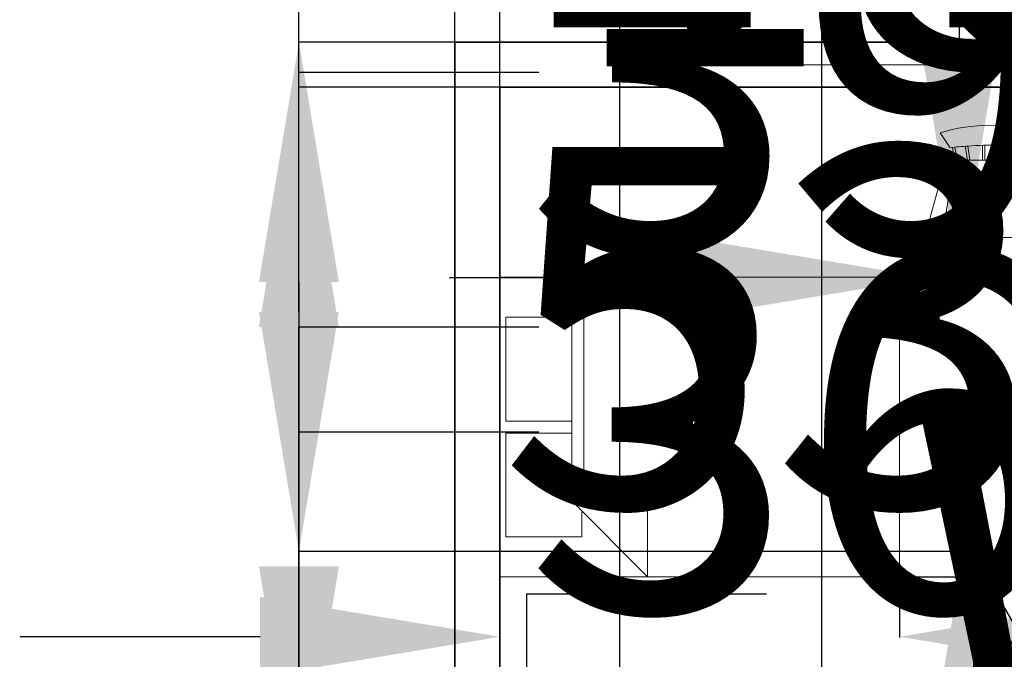
# Model space of a CAD drawing. Units: inches. Extents: x -307 to 2141, y -58 to 895.
# Tile 11 of 28: x 469 to 666, y 568 to 696. Entities that reach past the tile are written whole.
import ezdxf

# ---------------------------------------------------------------- set-up
doc = ezdxf.new("R2010")
doc.units = ezdxf.units.IN
doc.header["$MEASUREMENT"] = 0
for name, color, linetype, lineweight in [('A-ANNO-DIMS', 2, 'Continuous', 18), ('A-DOOR', 3, 'Continuous', 25), ('A-FURN', 8, 'Continuous', 18), ('A-GLAZ', 4, 'Continuous', 18), ('A-WALL', 7, 'Continuous', 35)]:
    doc.layers.add(name, color=color, linetype=linetype, lineweight=lineweight)
doc.styles.get("Standard").update_dxf_attribs({"font": 'arial.ttf'})
doc.dimstyles.get("Standard").update_dxf_attribs({"dimtxt": 72, "dimasz": 48, "dimexe": 0.18, "dimexo": 0.0625, "dimgap": 0.09, "dimtad": 0, "dimtih": 1, "dimtoh": 1, "dimdec": 0, "dimrnd": 48, "dimzin": 0, "dimdsep": 46, "dimlunit": 3, "dimtxsty": 'Standard', "dimcen": 0.09, "dimadec": 0, "dimazin": 0, "dimtfac": 1, "dimtdec": 0, "dimtofl": 0, "dimtmove": 0, "dimatfit": 3, "dimfxl": 1, "dimtolj": 1, "dimtzin": 0, "dimarcsym": 0})

# ---------------------------------------------------------------- blocks, each defined once
blk = doc.blocks.new('*U3')
for p, q in [((-40, 0), (-40, 6)), ((0, 0), (0, 6))]:
    blk.add_line(p, q)
blk.add_lwpolyline([(0, 0), (-34.64, -20), (-35.52, -18.48), (-0.88, 1.52)], close=True)
blk.add_arc((0, 0), 40, 180, 210)
blk = doc.blocks.new('Chair - Rocking')
for p, q in [((-8, -4.5), (-10, -1.5)), ((8, -4.5), (10, -1.5)), ((-7.5, -4.5), (-7, -7)), ((-6.5, -7), (-7.02225, -4.43)), ((-4.5, -7), (-4.96674, -4.19951)), ((-4, -7), (-4.40532, -4.16272)), ((-1.5, -4.05012), (-1.5, -7)), ((-1, -7), (-1, -4.05012)), ((1, -7), (1, -4.04655)), ((1.5, -4.05012), (1.5, -7)), ((4, -7), (4.40187, -4.18694)), ((4.5, -7), (4.96761, -4.19437)), ((6.5, -7), (7, -4.4057)), ((7.5, -4.5), (7, -7)), ((-9, -7.5), (-12, -18.49999)), ((-7, -7.5), (-9, -7.5)), ((-9, -18.49999), (-7, -7.5)), ((-8.23428, -6.99939), (-8.3093, -7.47958)), ((-8.23041, -7), (8.23915, -7)), ((7, -7.5), (9, -7.5)), ((9, -18.49999), (7, -7.5)), ((8.31071, -7.48854), (8.23449, -7.00073)), ((9, -7.5), (12, -18.49999)), ((-10.36644, -20.64523), (-10.5, -21.49999)), ((10.5, -21.49999), (10.3575, -20.58798)), ((-9, -22.49999), (-9.5, -26.49999)), ((0, -22.49999), (-9.5, -22.49999)), ((-8, -26.49999), (-7.5, -22.49999)), ((0, -22.49999), (9.5, -22.49999)), ((8, -26.49999), (7.5, -22.49999)), ((9, -22.49999), (9.5, -26.49999)), ((-9.5, -26.49999), (-8, -26.49999)), ((9.5, -26.49999), (8, -26.49999))]:
    blk.add_line(p, q)
for centre, radius, start, end in [((0, -34.08333), 34.08333, 72.93847, 107.0615), ((0, -68.25004), 64.25, 93.92211, 97.15267), ((0, -68.25004), 64.25, 82.84733, 93.92211), ((-10.5, -18.99999), 1.58114, 161.5651, 18.43495), ((10.5, -18.99999), 1.58114, 161.5651, 18.43495), ((-9.5, -21.49999), 1, 180, 270), ((9.5, -21.49999), 1, 270, 0)]:
    blk.add_arc(centre, radius, start, end)
blk = doc.blocks.new('Bed - Queen')
for p, q in [((0, -80.00003), (0, 0)), ((0, 0), (59.99999, 0)), ((59.99999, 0), (59.99999, -80.00003)), ((7.99999, -1.2), (28.79998, -1.2)), ((7.99999, -14.4), (7.99999, -1.2)), ((28.79998, -1.2), (28.79998, -14.4)), ((31.19999, -1.2), (51.99999, -1.2)), ((31.19999, -14.4), (31.19999, -1.2)), ((51.99999, -1.2), (51.99999, -16.4)), ((0, -14.4), (44.8, -14.4)), ((59.99999, -29.6), (44.8, -14.4)), ((44.8, -14.4), (44.8, -29.6)), ((44.8, -16.8), (0, -16.8)), ((51.99999, -16.4), (46.79936, -16.4)), ((44.8, -29.6), (59.99999, -29.6)), ((59.99999, -80.00003), (0, -80.00003))]:
    blk.add_line(p, q)
blk = doc.blocks.new('WIN-72IN')
blk.add_line((72, 4.5), (0, 4.5))
blk.add_lwpolyline([(72, 0), (0, 0), (0, 9), (72, 9)], close=True)
blk = doc.blocks.new('*D26')
at = {"layer": 'A-ANNO-DIMS', "color": 0, "lineweight": -2, "transparency": 16777216}
for p, q in [((565.34, 584.2), (565.34, 572.08)), ((645.34, 584.2), (645.34, 572.08)), ((517.34, 572.26), (469.34, 572.26)), ((693.34, 572.26), (741.34, 572.26))]:
    blk.add_line(p, q, dxfattribs=at)
at = {"layer": 'A-ANNO-DIMS', "color": 0, "transparency": 16777216}
for points in [[(517.34, 580.26), (517.34, 564.26), (565.34, 572.26)], [(693.34, 580.26), (693.34, 564.26), (645.34, 572.26)]]:
    blk.add_solid(points, dxfattribs=at)
at = {"layer": 'Defpoints', "color": 0, "transparency": 16777216}
for p in [(565.34, 584.26), (645.34, 584.26), (565.34, 572.26)]:
    blk.add_point(p, dxfattribs=at)
at = {"layer": 'A-ANNO-DIMS', "color": 0, "transparency": 16777216, "insert": (178.23, 572.26), "char_height": 72, "attachment_point": 5}
blk.add_mtext('\\A1;BED 80 TYP.', dxfattribs=at)
blk = doc.blocks.new('*D27')
at = {"layer": 'A-ANNO-DIMS', "color": 0, "lineweight": -2, "transparency": 16777216}
for p, q in [((657.34, 692.26), (657.34, 740.26)), ((645.4, 644.26), (657.52, 644.26)), ((645.4, 584.26), (657.52, 584.26)), ((657.34, 536.26), (657.34, 488.26)), ((657.34, 488.26), (609.34, 488.26))]:
    blk.add_line(p, q, dxfattribs=at)
at = {"layer": 'A-ANNO-DIMS', "color": 0, "transparency": 16777216}
for points in [[(649.34, 692.26), (665.34, 692.26), (657.34, 644.26)], [(649.34, 536.26), (665.34, 536.26), (657.34, 584.26)]]:
    blk.add_solid(points, dxfattribs=at)
at = {"layer": 'Defpoints', "color": 0, "transparency": 16777216}
for p in [(645.34, 644.26), (645.34, 584.26), (657.34, 584.26)]:
    blk.add_point(p, dxfattribs=at)
at = {"layer": 'A-ANNO-DIMS', "color": 0, "transparency": 16777216, "insert": (433.81, 488.26), "char_height": 72, "attachment_point": 5}
blk.add_mtext('\\A1;60 TYP.', dxfattribs=at)
blk = doc.blocks.new('*D30')
at = {"layer": 'A-ANNO-DIMS', "color": 0, "lineweight": -2, "transparency": 16777216}
for p, q in [((570.74, 532.83), (570.74, 580.83)), ((570.74, 580.83), (618.74, 580.83)), ((565.4, 484.83), (570.92, 484.83)), ((565.4, 448.83), (570.92, 448.83)), ((570.74, 400.83), (570.74, 352.83))]:
    blk.add_line(p, q, dxfattribs=at)
at = {"layer": 'A-ANNO-DIMS', "color": 0, "transparency": 16777216}
for points in [[(562.74, 532.83), (578.74, 532.83), (570.74, 484.83)], [(562.74, 400.83), (578.74, 400.83), (570.74, 448.83)]]:
    blk.add_solid(points, dxfattribs=at)
at = {"layer": 'Defpoints', "color": 0, "transparency": 16777216}
for p in [(565.34, 484.83), (570.74, 484.83), (565.34, 448.83)]:
    blk.add_point(p, dxfattribs=at)
at = {"layer": 'A-ANNO-DIMS', "color": 0, "transparency": 16777216, "insert": (1030.17, 580.83), "char_height": 72, "attachment_point": 5}
blk.add_mtext('\\A1;WINDOW 36 TYP.', dxfattribs=at)
blk = doc.blocks.new('*D36')
at = {"layer": 'A-ANNO-DIMS', "color": 0, "lineweight": -2, "transparency": 16777216}
for p, q in [((871.71, 562.4), (871.76, 610.4)), ((876.55, 514.4), (871.47, 514.4)), ((876.51, 481.35), (871.44, 481.36)), ((871.56, 433.36), (871.51, 385.36)), ((871.51, 385.36), (823.51, 385.36))]:
    blk.add_line(p, q, dxfattribs=at)
at = {"layer": 'A-ANNO-DIMS', "color": 0, "transparency": 16777216}
for points in [[(863.71, 562.41), (879.71, 562.4), (871.65, 514.4)], [(863.56, 433.37), (879.56, 433.35), (871.62, 481.36)]]:
    blk.add_solid(points, dxfattribs=at)
at = {"layer": 'Defpoints', "color": 0, "transparency": 16777216}
for p in [(876.61, 514.4), (871.62, 481.36), (876.57, 481.35)]:
    blk.add_point(p, dxfattribs=at)
at = {"layer": 'A-ANNO-DIMS', "color": 0, "transparency": 16777216, "insert": (548.95, 385.36), "char_height": 72, "attachment_point": 5}
blk.add_mtext('\\A1;WC 33 TYP.', dxfattribs=at)
blk = doc.blocks.new('*D37')
at = {"layer": 'A-ANNO-DIMS', "color": 0, "lineweight": -2, "transparency": 16777216}
for p, q in [((828.62, 519.41), (780.62, 519.46)), ((876.61, 514.46), (876.62, 519.54)), ((897.61, 514.44), (897.62, 519.51)), ((945.62, 519.28), (993.62, 519.22))]:
    blk.add_line(p, q, dxfattribs=at)
at = {"layer": 'A-ANNO-DIMS', "color": 0, "transparency": 16777216}
for points in [[(828.63, 527.41), (828.61, 511.41), (876.62, 519.36)], [(945.63, 527.28), (945.61, 511.28), (897.62, 519.33)]]:
    blk.add_solid(points, dxfattribs=at)
at = {"layer": 'Defpoints', "color": 0, "transparency": 16777216}
for p in [(876.62, 519.36), (876.61, 514.4), (897.61, 514.38)]:
    blk.add_point(p, dxfattribs=at)
at = {"layer": 'A-ANNO-DIMS', "color": 0, "transparency": 16777216, "insert": (604.68, 519.46), "char_height": 72, "attachment_point": 5}
blk.add_mtext('\\A1;21 TYP.', dxfattribs=at)
blk = doc.blocks.new('*D52')
at = {"layer": 'A-ANNO-DIMS', "color": 0, "lineweight": -2, "transparency": 16777216}
for p, q in [((660.21, 554.25), (660.21, 602.25)), ((673.8, 506.25), (660.03, 506.25)), ((673.8, 415.25), (660.03, 415.25)), ((660.21, 367.25), (660.21, 319.25))]:
    blk.add_line(p, q, dxfattribs=at)
at = {"layer": 'A-ANNO-DIMS', "color": 0, "transparency": 16777216}
for points in [[(652.21, 554.25), (668.21, 554.25), (660.21, 506.25)], [(652.21, 367.25), (668.21, 367.25), (660.21, 415.25)]]:
    blk.add_solid(points, dxfattribs=at)
at = {"layer": 'Defpoints', "color": 0, "transparency": 16777216}
for p in [(673.86, 506.25), (660.21, 415.25), (673.86, 415.25)]:
    blk.add_point(p, dxfattribs=at)
at = {"layer": 'A-ANNO-DIMS', "color": 0, "transparency": 16777216, "insert": (660.21, 460.75), "char_height": 72, "attachment_point": 5}
blk.add_mtext('\\A1;DINING SET 91', dxfattribs=at)
blk = doc.blocks.new('*D57')
at = {"layer": 'A-ANNO-DIMS', "color": 0, "lineweight": -2, "transparency": 16777216}
for p, q in [((651.25, 648.15), (651.25, 643.98)), ((675.68, 648.15), (675.68, 643.98)), ((603.25, 644.16), (555.25, 644.16)), ((723.68, 644.16), (771.68, 644.16))]:
    blk.add_line(p, q, dxfattribs=at)
at = {"layer": 'A-ANNO-DIMS', "color": 0, "transparency": 16777216}
for points in [[(603.25, 652.16), (603.25, 636.16), (651.25, 644.16)], [(723.68, 652.16), (723.68, 636.16), (675.68, 644.16)]]:
    blk.add_solid(points, dxfattribs=at)
at = {"layer": 'Defpoints', "color": 0, "transparency": 16777216}
for p in [(651.25, 648.21), (675.68, 648.21), (675.68, 644.16)]:
    blk.add_point(p, dxfattribs=at)
at = {"layer": 'A-ANNO-DIMS', "color": 0, "transparency": 16777216, "insert": (823.81, 644.16), "char_height": 72, "attachment_point": 5}
blk.add_mtext('\\A1;24', dxfattribs=at)
blk = doc.blocks.new('*D62')
at = {"layer": 'A-ANNO-DIMS', "color": 0, "lineweight": -2, "transparency": 16777216}
for p, q in [((556.34, 691.4), (556.34, 722.72)), ((604.34, 722.54), (656.85, 722.54)), ((868.34, 722.54), (815.82, 722.54)), ((916.34, 490.97), (916.34, 722.72))]:
    blk.add_line(p, q, dxfattribs=at)
at = {"layer": 'A-ANNO-DIMS', "color": 0, "transparency": 16777216}
for points in [[(604.34, 730.54), (604.34, 714.54), (556.34, 722.54)], [(868.34, 730.54), (868.34, 714.54), (916.34, 722.54)]]:
    blk.add_solid(points, dxfattribs=at)
at = {"layer": 'Defpoints', "color": 0, "transparency": 16777216}
for p in [(916.34, 722.54), (556.34, 691.34), (916.34, 490.9)]:
    blk.add_point(p, dxfattribs=at)
at = {"layer": 'A-ANNO-DIMS', "color": 0, "transparency": 16777216, "insert": (736.34, 722.54), "char_height": 72, "attachment_point": 5}
blk.add_mtext('\\A1;360', dxfattribs=at)
blk = doc.blocks.new('*D64')
at = {"layer": 'A-ANNO-DIMS', "color": 0, "lineweight": -2, "transparency": 16777216}
for p, q in [((556.27, 691.34), (524.95, 691.34)), ((525.13, 643.34), (525.13, 465.69)), ((525.13, 214.34), (525.13, 391.99)), ((556.27, 166.34), (524.95, 166.34))]:
    blk.add_line(p, q, dxfattribs=at)
at = {"layer": 'A-ANNO-DIMS', "color": 0, "transparency": 16777216}
for points in [[(517.13, 643.34), (533.13, 643.34), (525.13, 691.34)], [(517.13, 214.34), (533.13, 214.34), (525.13, 166.34)]]:
    blk.add_solid(points, dxfattribs=at)
at = {"layer": 'Defpoints', "color": 0, "transparency": 16777216}
for p in [(525.13, 691.34), (556.34, 691.34), (556.34, 166.34)]:
    blk.add_point(p, dxfattribs=at)
at = {"layer": 'A-ANNO-DIMS', "color": 0, "transparency": 16777216, "insert": (525.13, 428.84), "char_height": 72, "attachment_point": 5}
blk.add_mtext('\\A1;525', dxfattribs=at)
blk = doc.blocks.new('*D68')
at = {"layer": 'A-ANNO-DIMS', "color": 0, "lineweight": -2, "transparency": 16777216}
for p, q in [((525.13, 586.34), (525.13, 634.34)), ((525.13, 634.34), (573.13, 634.34)), ((565.27, 538.34), (524.95, 538.34)), ((556.27, 484.83), (524.95, 484.83)), ((525.13, 436.83), (525.13, 388.83))]:
    blk.add_line(p, q, dxfattribs=at)
at = {"layer": 'A-ANNO-DIMS', "color": 0, "transparency": 16777216}
for points in [[(517.13, 586.34), (533.13, 586.34), (525.13, 538.34)], [(517.13, 436.83), (533.13, 436.83), (525.13, 484.83)]]:
    blk.add_solid(points, dxfattribs=at)
at = {"layer": 'Defpoints', "color": 0, "transparency": 16777216}
for p in [(525.13, 538.34), (565.34, 538.34), (556.34, 484.83)]:
    blk.add_point(p, dxfattribs=at)
at = {"layer": 'A-ANNO-DIMS', "color": 0, "transparency": 16777216, "insert": (687.75, 634.34), "char_height": 72, "attachment_point": 5}
blk.add_mtext('\\A1;53.51', dxfattribs=at)
blk = doc.blocks.new('*D69')
at = {"layer": 'A-ANNO-DIMS', "color": 0, "lineweight": -2, "transparency": 16777216}
for p, q in [((525.13, 682.34), (525.13, 730.34)), ((525.13, 730.34), (573.13, 730.34)), ((565.27, 682.34), (524.95, 682.34)), ((525.13, 586.34), (525.13, 634.34)), ((565.27, 538.34), (524.95, 538.34))]:
    blk.add_line(p, q, dxfattribs=at)
at = {"layer": 'A-ANNO-DIMS', "color": 0, "transparency": 16777216}
for points in [[(517.13, 634.34), (533.13, 634.34), (525.13, 682.34)], [(517.13, 586.34), (533.13, 586.34), (525.13, 538.34)]]:
    blk.add_solid(points, dxfattribs=at)
at = {"layer": 'Defpoints', "color": 0, "transparency": 16777216}
for p in [(525.13, 682.34), (565.34, 682.34), (565.34, 538.34)]:
    blk.add_point(p, dxfattribs=at)
at = {"layer": 'A-ANNO-DIMS', "color": 0, "transparency": 16777216, "insert": (649.22, 730.34), "char_height": 72, "attachment_point": 5}
blk.add_mtext('\\A1;144', dxfattribs=at)
blk = doc.blocks.new('*D75')
at = {"layer": 'A-ANNO-DIMS', "color": 0, "lineweight": -2, "transparency": 16777216}
for p, q in [((565.34, 682.4), (565.34, 722.72)), ((613.34, 722.54), (637.34, 722.54)), ((685.34, 682.4), (685.34, 722.72)), ((685.34, 722.54), (733.34, 722.54))]:
    blk.add_line(p, q, dxfattribs=at)
at = {"layer": 'A-ANNO-DIMS', "color": 0, "transparency": 16777216}
for points in [[(613.34, 730.54), (613.34, 714.54), (565.34, 722.54)], [(637.34, 730.54), (637.34, 714.54), (685.34, 722.54)]]:
    blk.add_solid(points, dxfattribs=at)
at = {"layer": 'Defpoints', "color": 0, "transparency": 16777216}
for p in [(685.34, 722.54), (565.34, 682.34), (685.34, 682.34)]:
    blk.add_point(p, dxfattribs=at)
at = {"layer": 'A-ANNO-DIMS', "color": 0, "transparency": 16777216, "insert": (809.45, 722.54), "char_height": 72, "attachment_point": 5}
blk.add_mtext('\\A1;120', dxfattribs=at)
blk = doc.blocks.new('*D76')
at = {"layer": 'A-ANNO-DIMS', "color": 0, "lineweight": -2, "transparency": 16777216}
for p, q in [((646.34, 722.54), (598.34, 722.54)), ((694.34, 682.4), (694.34, 722.72)), ((778.34, 682.4), (778.34, 722.72)), ((826.34, 722.54), (874.34, 722.54))]:
    blk.add_line(p, q, dxfattribs=at)
at = {"layer": 'A-ANNO-DIMS', "color": 0, "transparency": 16777216}
for points in [[(646.34, 730.54), (646.34, 714.54), (694.34, 722.54)], [(826.34, 730.54), (826.34, 714.54), (778.34, 722.54)]]:
    blk.add_solid(points, dxfattribs=at)
at = {"layer": 'Defpoints', "color": 0, "transparency": 16777216}
for p in [(778.34, 722.54), (694.34, 682.34), (778.34, 682.34)]:
    blk.add_point(p, dxfattribs=at)
at = {"layer": 'A-ANNO-DIMS', "color": 0, "transparency": 16777216, "insert": (925.9, 722.54), "char_height": 72, "attachment_point": 5}
blk.add_mtext('\\A1;84', dxfattribs=at)
blk = doc.blocks.new('*D82')
at = {"layer": 'A-ANNO-DIMS', "color": 0, "lineweight": -2, "transparency": 16777216}
for p, q in [((525.13, 565.34), (525.13, 613.34)), ((525.13, 613.34), (573.13, 613.34)), ((802.27, 517.34), (524.95, 517.34)), ((802.27, 481.34), (524.95, 481.34)), ((525.13, 433.34), (525.13, 385.34))]:
    blk.add_line(p, q, dxfattribs=at)
at = {"layer": 'A-ANNO-DIMS', "color": 0, "transparency": 16777216}
for points in [[(517.13, 565.34), (533.13, 565.34), (525.13, 517.34)], [(517.13, 433.34), (533.13, 433.34), (525.13, 481.34)]]:
    blk.add_solid(points, dxfattribs=at)
at = {"layer": 'Defpoints', "color": 0, "transparency": 16777216}
for p in [(525.13, 517.34), (802.34, 517.34), (802.34, 481.34)]:
    blk.add_point(p, dxfattribs=at)
at = {"layer": 'A-ANNO-DIMS', "color": 0, "transparency": 16777216, "insert": (624.74, 613.34), "char_height": 72, "attachment_point": 5}
blk.add_mtext('\\A1;36', dxfattribs=at)
blk = doc.blocks.new('*D83')
at = {"layer": 'A-ANNO-DIMS', "color": 0, "lineweight": -2, "transparency": 16777216}
for p, q in [((947.54, 538.9), (947.54, 586.9)), ((916.4, 490.9), (947.72, 490.9)), ((907.4, 481.34), (947.72, 481.34)), ((947.54, 433.34), (947.54, 385.34)), ((947.54, 385.34), (899.54, 385.34))]:
    blk.add_line(p, q, dxfattribs=at)
at = {"layer": 'A-ANNO-DIMS', "color": 0, "transparency": 16777216}
for points in [[(939.54, 538.9), (955.54, 538.9), (947.54, 490.9)], [(939.54, 433.34), (955.54, 433.34), (947.54, 481.34)]]:
    blk.add_solid(points, dxfattribs=at)
at = {"layer": 'Defpoints', "color": 0, "transparency": 16777216}
for p in [(916.34, 490.9), (907.34, 481.34), (947.54, 481.34)]:
    blk.add_point(p, dxfattribs=at)
at = {"layer": 'A-ANNO-DIMS', "color": 0, "transparency": 16777216, "insert": (777.97, 385.34), "char_height": 72, "attachment_point": 5}
blk.add_mtext('\\A1;9.563', dxfattribs=at)
blk = doc.blocks.new('*D88')
at = {"layer": 'A-ANNO-DIMS', "color": 0, "lineweight": -2, "transparency": 16777216}
for p, q in [((517.33584, 722.544828), (469.33584, 722.544828)), ((565.33584, 295.403328), (565.33584, 722.724828)), ((754.33584, 271.403328), (754.33584, 722.724828)), ((802.33584, 722.544828), (850.33584, 722.544828))]:
    blk.add_line(p, q, dxfattribs=at)
at = {"layer": 'A-ANNO-DIMS', "color": 0, "transparency": 16777216}
for points in [[(517.33584, 730.544828), (517.33584, 714.544828), (565.33584, 722.544828)], [(802.33584, 730.544828), (802.33584, 714.544828), (754.33584, 722.544828)]]:
    blk.add_solid(points, dxfattribs=at)
at = {"layer": 'Defpoints', "color": 0, "transparency": 16777216}
for p in [(754.33584, 722.544828), (565.33584, 295.340828), (754.33584, 271.340828)]:
    blk.add_point(p, dxfattribs=at)
at = {"layer": 'A-ANNO-DIMS', "color": 0, "transparency": 16777216, "insert": (659.83584, 722.544828), "char_height": 72, "attachment_point": 5}
blk.add_mtext('\\A1;189', dxfattribs=at)
blk = doc.blocks.new('*D94')
at = {"layer": 'A-ANNO-DIMS', "color": 0, "lineweight": -2, "transparency": 16777216}
for p, q in [((517.34, 722.54), (469.34, 722.54)), ((565.34, 529.4), (565.34, 722.72)), ((629.84, 529.4), (629.84, 722.72)), ((677.84, 722.54), (725.84, 722.54))]:
    blk.add_line(p, q, dxfattribs=at)
at = {"layer": 'A-ANNO-DIMS', "color": 0, "transparency": 16777216}
for points in [[(517.34, 730.54), (517.34, 714.54), (565.34, 722.54)], [(677.84, 730.54), (677.84, 714.54), (629.84, 722.54)]]:
    blk.add_solid(points, dxfattribs=at)
at = {"layer": 'Defpoints', "color": 0, "transparency": 16777216}
for p in [(629.84, 722.54), (565.34, 529.34), (629.84, 529.34)]:
    blk.add_point(p, dxfattribs=at)
at = {"layer": 'A-ANNO-DIMS', "color": 0, "transparency": 16777216, "insert": (819.9, 722.54), "char_height": 72, "attachment_point": 5}
blk.add_mtext('\\A1;64.5', dxfattribs=at)
blk = doc.blocks.new('*D95')
at = {"layer": 'A-ANNO-DIMS', "color": 0, "lineweight": -2, "transparency": 16777216}
for p, q in [((947.54, 577.34), (947.54, 625.34)), ((947.54, 625.34), (995.54, 625.34)), ((629.9, 529.34), (947.72, 529.34)), ((629.9, 502.66), (947.72, 502.66)), ((947.54, 454.66), (947.54, 406.66))]:
    blk.add_line(p, q, dxfattribs=at)
at = {"layer": 'A-ANNO-DIMS', "color": 0, "transparency": 16777216}
for points in [[(939.54, 577.34), (955.54, 577.34), (947.54, 529.34)], [(939.54, 454.66), (955.54, 454.66), (947.54, 502.66)]]:
    blk.add_solid(points, dxfattribs=at)
at = {"layer": 'Defpoints', "color": 0, "transparency": 16777216}
for p in [(629.84, 529.34), (947.54, 529.34), (629.84, 502.66)]:
    blk.add_point(p, dxfattribs=at)
at = {"layer": 'A-ANNO-DIMS', "color": 0, "transparency": 16777216, "insert": (1117.8, 625.34), "char_height": 72, "attachment_point": 5}
blk.add_mtext('\\A1;26.68', dxfattribs=at)
blk = doc.blocks.new('*D96')
at = {"layer": 'A-ANNO-DIMS', "color": 0, "lineweight": -2, "transparency": 16777216}
for p, q in [((646.34, 722.54), (598.34, 722.54)), ((694.34, 598.4), (694.34, 722.72)), ((730.34, 598.4), (730.34, 722.72)), ((778.34, 722.54), (826.34, 722.54))]:
    blk.add_line(p, q, dxfattribs=at)
at = {"layer": 'A-ANNO-DIMS', "color": 0, "transparency": 16777216}
for points in [[(646.34, 730.54), (646.34, 714.54), (694.34, 722.54)], [(778.34, 730.54), (778.34, 714.54), (730.34, 722.54)]]:
    blk.add_solid(points, dxfattribs=at)
at = {"layer": 'Defpoints', "color": 0, "transparency": 16777216}
for p in [(730.34, 722.54), (694.34, 598.34), (730.34, 598.34)]:
    blk.add_point(p, dxfattribs=at)
at = {"layer": 'A-ANNO-DIMS', "color": 0, "transparency": 16777216, "insert": (877.95, 722.54), "char_height": 72, "attachment_point": 5}
blk.add_mtext('\\A1;36', dxfattribs=at)
blk = doc.blocks.new('*D98')
at = {"layer": 'A-ANNO-DIMS', "color": 0, "lineweight": -2, "transparency": 16777216}
for p, q in [((525.13, 637.34), (525.13, 685.34)), ((525.13, 685.34), (573.13, 685.34)), ((787.27, 589.34), (524.95, 589.34)), ((787.27, 550.34), (524.95, 550.34)), ((525.13, 502.34), (525.13, 454.34))]:
    blk.add_line(p, q, dxfattribs=at)
at = {"layer": 'A-ANNO-DIMS', "color": 0, "transparency": 16777216}
for points in [[(517.13, 637.34), (533.13, 637.34), (525.13, 589.34)], [(517.13, 502.34), (533.13, 502.34), (525.13, 550.34)]]:
    blk.add_solid(points, dxfattribs=at)
at = {"layer": 'Defpoints', "color": 0, "transparency": 16777216}
for p in [(525.13, 589.34), (787.34, 589.34), (787.34, 550.34)]:
    blk.add_point(p, dxfattribs=at)
at = {"layer": 'A-ANNO-DIMS', "color": 0, "transparency": 16777216, "insert": (624.84, 685.34), "char_height": 72, "attachment_point": 5}
blk.add_mtext('\\A1;39', dxfattribs=at)
blk = doc.blocks.new('*D101')
at = {"layer": 'A-ANNO-DIMS', "color": 0, "lineweight": -2, "transparency": 16777216}
for p, q in [((508.34, 722.54), (460.34, 722.54)), ((556.34, 691.4), (556.34, 722.72)), ((589.36, 691.4), (589.36, 722.72)), ((637.36, 722.54), (685.36, 722.54))]:
    blk.add_line(p, q, dxfattribs=at)
at = {"layer": 'A-ANNO-DIMS', "color": 0, "transparency": 16777216}
for points in [[(508.34, 730.54), (508.34, 714.54), (556.34, 722.54)], [(637.36, 730.54), (637.36, 714.54), (589.36, 722.54)]]:
    blk.add_solid(points, dxfattribs=at)
at = {"layer": 'Defpoints', "color": 0, "transparency": 16777216}
for p in [(589.36, 722.54), (556.34, 691.34), (589.36, 691.34)]:
    blk.add_point(p, dxfattribs=at)
at = {"layer": 'A-ANNO-DIMS', "color": 0, "transparency": 16777216, "insert": (806.54, 722.54), "char_height": 72, "attachment_point": 5}
blk.add_mtext('\\A1;33.02', dxfattribs=at)
blk = doc.blocks.new('*D103')
at = {"layer": 'A-ANNO-DIMS', "color": 0, "lineweight": -2, "transparency": 16777216}
for p, q in [((637.34, 722.54), (589.34, 722.54)), ((685.34, 682.4), (685.34, 722.72)), ((694.34, 682.4), (694.34, 722.72)), ((742.34, 722.54), (790.34, 722.54))]:
    blk.add_line(p, q, dxfattribs=at)
at = {"layer": 'A-ANNO-DIMS', "color": 0, "transparency": 16777216}
for points in [[(637.34, 730.54), (637.34, 714.54), (685.34, 722.54)], [(742.34, 730.54), (742.34, 714.54), (694.34, 722.54)]]:
    blk.add_solid(points, dxfattribs=at)
at = {"layer": 'Defpoints', "color": 0, "transparency": 16777216}
for p in [(694.34, 722.54), (685.34, 682.34), (694.34, 682.34)]:
    blk.add_point(p, dxfattribs=at)
at = {"layer": 'A-ANNO-DIMS', "color": 0, "transparency": 16777216, "insert": (814.1, 722.54), "char_height": 72, "attachment_point": 5}
blk.add_mtext('\\A1;9', dxfattribs=at)
blk = doc.blocks.new('*D107')
at = {"layer": 'A-ANNO-DIMS', "color": 0, "lineweight": -2, "transparency": 16777216}
for p, q in [((517.34, 722.54), (469.34, 722.54)), ((565.34, 409.4), (565.34, 722.72)), ((589.34, 409.4), (589.34, 722.72)), ((637.34, 722.54), (685.34, 722.54))]:
    blk.add_line(p, q, dxfattribs=at)
at = {"layer": 'A-ANNO-DIMS', "color": 0, "transparency": 16777216}
for points in [[(517.34, 730.54), (517.34, 714.54), (565.34, 722.54)], [(637.34, 730.54), (637.34, 714.54), (589.34, 722.54)]]:
    blk.add_solid(points, dxfattribs=at)
at = {"layer": 'Defpoints', "color": 0, "transparency": 16777216}
for p in [(589.34, 722.54), (565.34, 409.34), (589.34, 409.34)]:
    blk.add_point(p, dxfattribs=at)
at = {"layer": 'A-ANNO-DIMS', "color": 0, "transparency": 16777216, "insert": (835.49, 722.54), "char_height": 72, "attachment_point": 5}
blk.add_mtext('\\A1;24.003', dxfattribs=at)
blk = doc.blocks.new('*D108')
at = {"layer": 'A-ANNO-DIMS', "color": 0, "lineweight": -2, "transparency": 16777216}
for p, q in [((947.54, 550.66), (947.54, 598.66)), ((589.4, 502.66), (947.72, 502.66)), ((589.4, 409.34), (947.72, 409.34)), ((947.54, 361.34), (947.54, 313.34))]:
    blk.add_line(p, q, dxfattribs=at)
at = {"layer": 'A-ANNO-DIMS', "color": 0, "transparency": 16777216}
for points in [[(939.54, 550.66), (955.54, 550.66), (947.54, 502.66)], [(939.54, 361.34), (955.54, 361.34), (947.54, 409.34)]]:
    blk.add_solid(points, dxfattribs=at)
at = {"layer": 'Defpoints', "color": 0, "transparency": 16777216}
for p in [(589.34, 502.66), (947.54, 502.66), (589.34, 409.34)]:
    blk.add_point(p, dxfattribs=at)
at = {"layer": 'A-ANNO-DIMS', "color": 0, "transparency": 16777216, "insert": (947.54, 456), "char_height": 72, "attachment_point": 5}
blk.add_mtext('\\A1;93.32', dxfattribs=at)

msp = doc.modelspace()

# ---------------------------------------------------------------- linework, layer by layer
at = {"layer": 'A-WALL'}
for p, q in [((916.3358, 691.3408), (556.3358, 691.3408)), ((556.3358, 691.3408), (556.3358, 91.3408)), ((907.3358, 682.3408), (565.3358, 682.3408)), ((565.3358, 682.3408), (565.3358, 100.3408))]:
    msp.add_line(p, q, dxfattribs=at)

# ---------------------------------------------------------------- block references
at = {"layer": 'A-DOOR', "xscale": 1.272826874134829, "yscale": 1.272826874134829, "zscale": 1.272826874134829, "rotation": 270}
msp.add_blockref('*U3', (686.6989, 538.3408), dxfattribs=at)
at = {"layer": 'A-FURN'}
msp.add_blockref('Chair - Rocking', (663.4642, 674.711), dxfattribs=at)
at = {"layer": 'A-FURN', "xscale": -1, "rotation": 90}
msp.add_blockref('Bed - Queen', (565.3358, 644.2648), dxfattribs=at)
at = {"layer": 'A-GLAZ'}
msp.add_blockref('WIN-72IN', (589.3575, 682.341), dxfattribs=at)

# ---------------------------------------------------------------- dimensions: what is measured, and where the dimension line sits
at = {"layer": 'A-ANNO-DIMS'}
for base, p1, p2, override, picture, middle in [((525.1318, 682.3408), (565.3358, 538.3408), (565.3358, 682.3408), {"dimdec": 0, "dimlfac": 1, "dimrnd": 0, "dimzin": 0, "dimdsep": 46, "dimlunit": 2}, '*D69', (649.2246, 730.3408)), ((525.1318, 589.3408), (787.3358, 550.3408), (787.3358, 589.3408), {"dimdec": 0, "dimlfac": 1, "dimrnd": 0, "dimzin": 0, "dimdsep": 46, "dimlunit": 2}, '*D98', (624.8398, 685.3408)), ((525.1318, 691.3408), (556.3358, 166.3408), (556.3358, 691.3408), {"dimdec": 0, "dimlfac": 1, "dimrnd": 0, "dimzin": 0, "dimdsep": 46, "dimlunit": 2}, '*D64', (525.1318, 428.8408)), ((525.1318, 538.3408), (556.3358, 484.8333), (565.3358, 538.3408), {"dimdec": 2, "dimlfac": 1, "dimrnd": 0, "dimzin": 0, "dimdsep": 46, "dimlunit": 2}, '*D68', (687.7539, 634.3408)), ((947.5398, 529.3408), (629.8358, 502.6632), (629.8358, 529.3408), {"dimdec": 2, "dimlfac": 1, "dimrnd": 0, "dimzin": 0, "dimdsep": 46, "dimlunit": 2}, '*D95', (1117.799, 625.3408)), ((525.1318, 517.3408), (802.3358, 481.3408), (802.3358, 517.3408), {"dimdec": 0, "dimlfac": 1, "dimrnd": 0, "dimzin": 0, "dimdsep": 46, "dimlunit": 2}, '*D82', (624.7416, 613.3408)), ((947.5398, 502.6632), (589.339, 409.3408), (589.339, 502.6632), {"dimdec": 2, "dimlfac": 1, "dimrnd": 0, "dimzin": 0, "dimdsep": 46, "dimlunit": 2}, '*D108', (947.5398, 456.002)), ((947.5398, 481.3408), (916.3358, 490.9034), (907.3358, 481.3408), {"dimdec": 3, "dimlfac": 1, "dimrnd": 0, "dimzin": 0, "dimdsep": 46, "dimlunit": 2}, '*D83', (777.9683, 385.3408))]:
    dim = msp.add_linear_dim(base=base, p1=p1, p2=p2, angle=90, dimstyle='Standard', override=override, dxfattribs=at)
    dim.commit()
    dim.dimension.update_dxf_attribs({"geometry": picture, "text_midpoint": middle})
for base, p1, p2, override, picture, middle in [((589.3579, 722.5448), (556.3358, 691.3408), (589.3579, 691.3408), {"dimdec": 2, "dimlfac": 1, "dimrnd": 0, "dimzin": 0, "dimdsep": 46, "dimlunit": 2}, '*D101', (806.5366, 722.5448)), ((754.3358, 722.5448), (565.3358, 295.3408), (754.3358, 271.3408), {"dimdec": 0, "dimlfac": 1, "dimrnd": 0, "dimzin": 0, "dimdsep": 46, "dimlunit": 2}, '*D88', (659.8358, 722.5448)), ((629.8358, 722.5448), (565.3358, 529.3408), (629.8358, 529.3408), {"dimdec": 1, "dimlfac": 1, "dimrnd": 0, "dimzin": 0, "dimdsep": 46, "dimlunit": 2}, '*D94', (819.904, 722.5448)), ((589.339, 722.5448), (565.3358, 409.3408), (589.339, 409.3408), {"dimdec": 3, "dimlfac": 1, "dimrnd": 0, "dimzin": 0, "dimdsep": 46, "dimlunit": 2}, '*D107', (835.4945, 722.5448)), ((916.3358, 722.5448), (556.3358, 691.3408), (916.3358, 490.9034), {"dimdec": 0, "dimlfac": 1, "dimrnd": 0, "dimzin": 0, "dimdsep": 46, "dimlunit": 2}, '*D62', (736.3358, 722.5448)), ((685.3358, 722.5448), (565.3358, 682.3408), (685.3358, 682.3408), {"dimdec": 0, "dimlfac": 1, "dimrnd": 0, "dimzin": 0, "dimdsep": 46, "dimlunit": 2}, '*D75', (809.4531, 722.5448)), ((694.3358, 722.5448), (685.3358, 682.3408), (694.3358, 682.3408), {"dimdec": 0, "dimlfac": 1, "dimrnd": 0, "dimzin": 0, "dimdsep": 46, "dimlunit": 2}, '*D103', (814.0984, 722.5448)), ((778.3358, 722.5448), (694.3358, 682.3408), (778.3358, 682.3408), {"dimdec": 0, "dimlfac": 1, "dimrnd": 0, "dimzin": 0, "dimdsep": 46, "dimlunit": 2}, '*D76', (925.8965, 722.5448)), ((730.3358, 722.5448), (694.3358, 598.3408), (730.3358, 598.3408), {"dimdec": 0, "dimlfac": 1, "dimrnd": 0, "dimzin": 0, "dimdsep": 46, "dimlunit": 2}, '*D96', (877.9456, 722.5448)), ((675.6817, 644.161), (651.2466, 648.211), (675.6817, 648.211), {"dimdec": 0, "dimlfac": 1, "dimrnd": 0, "dimzin": 0, "dimdsep": 46, "dimlunit": 2}, '*D57', (823.8072, 644.161))]:
    dim = msp.add_linear_dim(base=base, p1=p1, p2=p2, dimstyle='Standard', override=override, dxfattribs=at)
    dim.commit()
    dim.dimension.update_dxf_attribs({"geometry": picture, "text_midpoint": middle})
for base, p1, p2, angle, text, picture, middle in [((570.7358, 484.8333), (565.3358, 448.8333), (565.3358, 484.8333), 90, 'WINDOW <> TYP.', '*D30', (1030.1737, 580.8333)), ((565.3358, 572.2648), (645.3359, 584.2648), (565.3358, 584.2648), 180, 'BED <> TYP.', '*D26', (178.2254, 572.2648)), ((657.3359, 584.2648), (645.3359, 644.2648), (645.3359, 584.2648), 270, '<> TYP.', '*D27', (433.8134, 488.2648)), ((660.2083, 415.2485), (673.8583, 506.2485), (673.8583, 415.2485), 270, 'DINING SET <>', '*D52', (660.2083, 460.7485)), ((876.6162, 519.3557), (897.6106, 514.3753), (876.6106, 514.3988), 179.935892, '<> TYP.', '*D37', (604.6763, 519.4631)), ((871.6167, 481.3581), (876.6106, 514.3988), (876.5736, 481.3526), 269.935892, 'WC <> TYP.', '*D36', (548.95, 385.3582))]:
    dim = msp.add_linear_dim(base=base, p1=p1, p2=p2, angle=angle, text=text, dimstyle='Standard', override={"dimdec": 0, "dimlfac": 1, "dimrnd": 0, "dimzin": 0, "dimdsep": 46, "dimlunit": 2}, dxfattribs=at)
    dim.commit()
    dim.dimension.update_dxf_attribs({"geometry": picture, "text_midpoint": middle})

doc.saveas('drawing.dxf')
